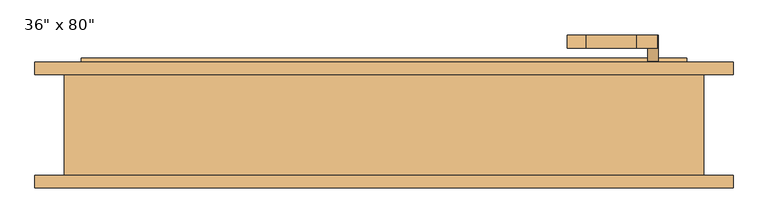
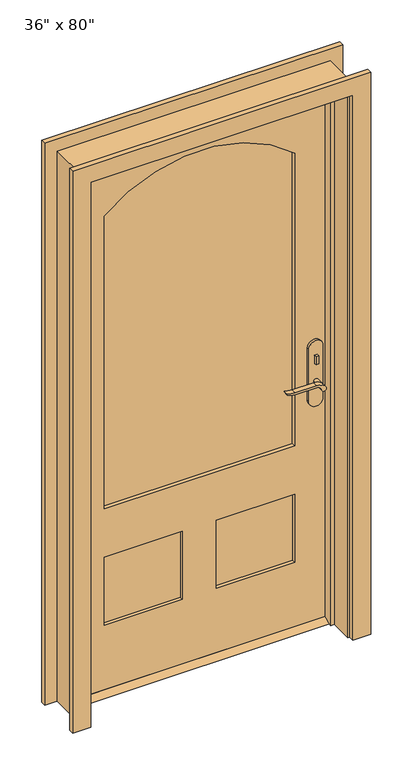
"""IFC4 building model written with IfcOpenShell, lengths in millimetres: door geometry."""

from ifc_helpers import new_model, si_unit, point, frame, frame_2d, origin, place, context, project, spatial, polyline, circle_curve, trimmed, segment, composite_curve, outline, extrude, faceted_brep, source, transform, mapped, element, save


def door_808aeb8e(model_context):
    return source(origin(), model_context, "Body", "SolidModel", [
        extrude(outline(polyline([(38.1, 12.7), (73.025, 12.7), (98.425, 0.0), (12.7, 0.0), (38.1, 12.7)])), frame((-457.2, 0.0, 0.0), z_axis=(1.0, 0.0, 0.0), x_axis=(0.0, 1.0, 0.0)), (0.0, 0.0, 1.0), 914.4),
        extrude(outline(polyline([(411.4, 18.1), (401.4, 18.1), (401.4, 28.1), (411.4, 28.1), (411.4, 18.1)])), frame((0.0, 0.0, 981.9), z_axis=(0.0, 0.0, 1.0), x_axis=(1.0, 0.0, 0.0)), (0.0, 0.0, 1.0), 30.0),
        extrude(outline(composite_curve([segment(trimmed(circle_curve(frame_2d((996.9, 406.4)), 8.0), [point((996.9, 398.4))], [point((996.9, 414.4))], False, "CARTESIAN"), True, "CONTINUOUS"), segment(trimmed(circle_curve(frame_2d((996.9, 406.4)), 8.0), [point((996.9, 414.4))], [point((996.9, 398.4))], False, "CARTESIAN"), True, "CONTINUOUS")], self_intersect=False)), frame((0.0, 83.025, 0.0), z_axis=(0.0, 1.0, 0.0), x_axis=(0.0, 0.0, 1.0)), (0.0, 0.0, 1.0), 10.0),
        extrude(outline(composite_curve([segment(trimmed(circle_curve(frame_2d((897.1555521, 382.7324871)), 37.2832219), [point((919.0523287, 412.9081363))], [point((934.4, 381.0325667))], False, "CARTESIAN"), True, "CONTINUOUS"), segment(polyline([(934.4, 381.0325667), (934.4, 304.7564091)]), True, "CONTINUOUS"), segment(trimmed(circle_curve(frame_2d((1017.6850638, 304.8227909)), 83.2850902), [point((934.4, 304.7564091))], [point((939.4, 276.4))], True, "CARTESIAN"), True, "CONTINUOUS"), segment(polyline([(939.4, 276.4), (936.6135558, 276.4)]), True, "CONTINUOUS"), segment(trimmed(circle_curve(frame_2d((986.6709207, 308.3396612)), 59.3791355), [point((936.6135558, 276.4))], [point((927.4, 304.7564091))], False, "CARTESIAN"), True, "CONTINUOUS"), segment(polyline([(927.4, 304.7564091), (927.4, 381.0138099)]), True, "CONTINUOUS"), segment(trimmed(circle_curve(frame_2d((909.2738613, 381.0138099)), 18.1261387), [point((927.4, 381.0138099))], [point((914.4, 398.4))], True, "CARTESIAN"), True, "CONTINUOUS"), segment(trimmed(circle_curve(frame_2d((914.4, 406.4)), 8.0), [point((914.4, 398.4))], [point((919.0523287, 412.9081363))], False, "CARTESIAN"), True, "CONTINUOUS")], self_intersect=False)), frame((0.0, -21.9, 0.0), z_axis=(0.0, 1.0, 0.0), x_axis=(0.0, 0.0, 1.0)), (0.0, 0.0, 1.0), 20.0),
        extrude(outline(composite_curve([segment(trimmed(circle_curve(frame_2d((914.4, 406.4)), 8.0), [point((914.3999903, 398.4))], [point((919.0523287, 412.9081363))], False, "CARTESIAN"), True, "CONTINUOUS"), segment(trimmed(circle_curve(frame_2d((897.1555521, 382.7324871)), 37.2832219), [point((919.0523287, 412.9081363))], [point((934.4, 381.0325667))], False, "CARTESIAN"), True, "CONTINUOUS"), segment(polyline([(934.4, 381.0325667), (934.4, 304.7564091)]), True, "CONTINUOUS"), segment(trimmed(circle_curve(frame_2d((1017.6850638, 304.8227909)), 83.2850902), [point((934.4, 304.7564091))], [point((939.4, 276.4))], True, "CARTESIAN"), True, "CONTINUOUS"), segment(polyline([(939.4, 276.4), (936.6135558, 276.4)]), True, "CONTINUOUS"), segment(trimmed(circle_curve(frame_2d((986.6709207, 308.3396612)), 59.3791355), [point((936.6135558, 276.4))], [point((927.4, 304.7564091))], False, "CARTESIAN"), True, "CONTINUOUS"), segment(polyline([(927.4, 304.7564091), (927.4, 381.0138122)]), True, "CONTINUOUS"), segment(trimmed(circle_curve(frame_2d((909.2738682, 381.0138122)), 18.1261318), [point((927.4, 381.0138122))], [point((914.3999903, 398.4))], True, "CARTESIAN"), True, "CONTINUOUS")], self_intersect=False)), frame((0.0, 113.025, 0.0), z_axis=(0.0, 1.0, 0.0), x_axis=(0.0, 0.0, 1.0)), (0.0, 0.0, 1.0), 20.0),
        extrude(outline(composite_curve([segment(trimmed(circle_curve(frame_2d((914.4, 406.4)), 8.0), [point((914.4, 398.4))], [point((914.4, 414.4))], False, "CARTESIAN"), True, "CONTINUOUS"), segment(trimmed(circle_curve(frame_2d((914.4, 406.4)), 8.0), [point((914.4, 414.4))], [point((914.4, 398.4))], False, "CARTESIAN"), True, "CONTINUOUS")], self_intersect=False)), frame((0.0, -1.9, 0.0), z_axis=(0.0, 1.0, 0.0), x_axis=(0.0, 0.0, 1.0)), (0.0, 0.0, 1.0), 30.0),
        extrude(outline(composite_curve([segment(trimmed(circle_curve(frame_2d((914.4, 406.4)), 8.0), [point((914.4, 398.4))], [point((914.4, 414.4))], False, "CARTESIAN"), True, "CONTINUOUS"), segment(trimmed(circle_curve(frame_2d((914.4, 406.4)), 8.0), [point((914.4, 414.4))], [point((914.4, 398.4))], False, "CARTESIAN"), True, "CONTINUOUS")], self_intersect=False)), frame((0.0, 83.025, 0.0), z_axis=(0.0, 1.0, 0.0), x_axis=(0.0, 0.0, 1.0)), (0.0, 0.0, 1.0), 30.0),
        extrude(outline(composite_curve([segment(polyline([(844.4, 431.4), (1039.4, 431.4)]), True, "CONTINUOUS"), segment(trimmed(circle_curve(frame_2d((1039.4, 406.4)), 25.0), [point((1039.4, 431.4))], [point((1039.4, 381.4))], False, "CARTESIAN"), True, "CONTINUOUS"), segment(polyline([(1039.4, 381.4), (844.4, 381.4)]), True, "CONTINUOUS"), segment(trimmed(circle_curve(frame_2d((844.4, 406.4)), 25.0), [point((844.4, 381.4))], [point((844.4, 431.4))], False, "CARTESIAN"), True, "CONTINUOUS")], self_intersect=False)), frame((0.0, 28.1, 0.0), z_axis=(0.0, 1.0, 0.0), x_axis=(0.0, 0.0, 1.0)), (0.0, 0.0, 1.0), 10.0),
        extrude(outline(composite_curve([segment(polyline([(844.4, 431.4), (1039.4, 431.4)]), True, "CONTINUOUS"), segment(trimmed(circle_curve(frame_2d((1039.4, 406.4)), 25.0), [point((1039.4, 431.4))], [point((1039.4, 381.4))], False, "CARTESIAN"), True, "CONTINUOUS"), segment(polyline([(1039.4, 381.4), (844.4, 381.4)]), True, "CONTINUOUS"), segment(trimmed(circle_curve(frame_2d((844.4, 406.4)), 25.0), [point((844.4, 381.4))], [point((844.4, 431.4))], False, "CARTESIAN"), True, "CONTINUOUS")], self_intersect=False)), frame((0.0, 73.025, 0.0), z_axis=(0.0, 1.0, 0.0), x_axis=(0.0, 0.0, 1.0)), (0.0, 0.0, 1.0), 10.0),
        extrude(outline(polyline([(2032.0, -457.2), (12.7, -457.2), (12.7, 457.2), (2032.0, 457.2), (2032.0, -457.2)]), holes=[composite_curve([segment(polyline([(688.975, -336.55), (1784.35, -336.55)]), True, "CONTINUOUS"), segment(trimmed(circle_curve(frame_2d((1401.92125, 0.0)), 509.42875), [point((1784.35, -336.55))], [point((1784.35, 336.55))], True, "CARTESIAN"), True, "CONTINUOUS"), segment(polyline([(1784.35, 336.55), (688.975, 336.55), (688.975, -336.55)]), True, "CONTINUOUS")], self_intersect=False), polyline([(508.0, -60.325), (254.0, -60.325), (254.0, -336.55), (508.0, -336.55), (508.0, -60.325)]), polyline([(508.0, 336.55), (254.0, 336.55), (254.0, 60.325), (508.0, 60.325), (508.0, 336.55)])]), frame((0.0, 38.1, 0.0), z_axis=(0.0, 1.0, 0.0), x_axis=(0.0, 0.0, 1.0)), (0.0, 0.0, 1.0), 34.925),
        faceted_brep([(482.6, 73.025, 0.0), (482.6, -79.375, 0.0), (457.2, -79.375, 0.0), (457.2, 3.175, 0.0), (444.5, 3.175, 0.0), (444.5, 38.1, 0.0), (457.2, 38.1, 0.0), (457.2, 73.025, 0.0), (482.6, 73.025, 2057.4), (482.6, -79.375, 2057.4), (-482.6, -79.375, 2057.4), (-482.6, -79.375, 0.0), (-457.2, -79.375, 0.0), (-457.2, -79.375, 2032.0), (457.2, -79.375, 2032.0), (457.2, 3.175, 2032.0), (-457.2, 3.175, 2032.0), (-457.2, 3.175, 0.0), (-444.5, 3.175, 0.0), (-444.5, 3.175, 2019.3), (444.5, 3.175, 2019.3), (444.5, 38.1, 2019.3), (-444.5, 38.1, 2019.3), (-444.5, 38.1, 0.0), (-457.2, 38.1, 0.0), (-457.2, 38.1, 2032.0), (457.2, 38.1, 2032.0), (457.2, 73.025, 2032.0), (-457.2, 73.025, 2032.0), (-457.2, 73.025, 0.0), (-482.6, 73.025, 0.0), (-482.6, 73.025, 2057.4)], [[[0, 1, 2, 3, 4, 5, 6, 7]], [[1, 0, 8, 9]], [[2, 1, 9, 10, 11, 12, 13, 14]], [[3, 2, 14, 15]], [[4, 3, 15, 16, 17, 18, 19, 20]], [[5, 4, 20, 21]], [[6, 5, 21, 22, 23, 24, 25, 26]], [[7, 6, 26, 27]], [[0, 7, 27, 28, 29, 30, 31, 8]], [[9, 8, 31, 10]], [[15, 14, 13, 16]], [[21, 20, 19, 22]], [[27, 26, 25, 28]], [[30, 29, 24, 23, 18, 17, 12, 11]], [[10, 31, 30, 11]], [[16, 13, 12, 17]], [[22, 19, 18, 23]], [[28, 25, 24, 29]]]),
        extrude(outline(polyline([(-60.325, 49.7416667), (-336.55, 49.7416667), (-336.55, 61.3833333), (-60.325, 61.3833333), (-60.325, 49.7416667)])), frame((0.0, 0.0, 254.0), z_axis=(0.0, 0.0, 1.0), x_axis=(1.0, 0.0, 0.0)), (0.0, 0.0, 1.0), 254.0),
        extrude(outline(polyline([(336.55, 49.7416667), (60.325, 49.7416667), (60.325, 61.3833333), (336.55, 61.3833333), (336.55, 49.7416667)])), frame((0.0, 0.0, 254.0), z_axis=(0.0, 0.0, 1.0), x_axis=(1.0, 0.0, 0.0)), (0.0, 0.0, 1.0), 254.0),
        extrude(outline(composite_curve([segment(polyline([(688.975, -336.55), (688.975, 336.55), (1784.35, 336.55)]), True, "CONTINUOUS"), segment(trimmed(circle_curve(frame_2d((1401.92125, 0.0)), 509.42875), [point((1784.35, 336.55))], [point((1784.35, -336.55))], False, "CARTESIAN"), True, "CONTINUOUS"), segment(polyline([(1784.35, -336.55), (688.975, -336.55)]), True, "CONTINUOUS")], self_intersect=False)), frame((0.0, 52.07, 0.0), z_axis=(0.0, 1.0, 0.0), x_axis=(0.0, 0.0, 1.0)), (0.0, 0.0, 1.0), 6.985),
        extrude(outline(polyline([(0.0, -527.05), (0.0, -463.55), (2038.35, -463.55), (2038.35, 463.55), (0.0, 463.55), (0.0, 527.05), (2101.85, 527.05), (2101.85, -527.05), (0.0, -527.05)])), frame((0.0, -98.425, 0.0), z_axis=(0.0, 1.0, 0.0), x_axis=(0.0, 0.0, 1.0)), (0.0, 0.0, 1.0), 19.05),
        extrude(outline(polyline([(0.0, -527.05), (0.0, -463.55), (2038.35, -463.55), (2038.35, 463.55), (0.0, 463.55), (0.0, 527.05), (2101.85, 527.05), (2101.85, -527.05), (0.0, -527.05)])), frame((0.0, 73.025, 0.0), z_axis=(0.0, 1.0, 0.0), x_axis=(0.0, 0.0, 1.0)), (0.0, 0.0, 1.0), 19.05),
    ])


if __name__ == "__main__":
    model = new_model("IFC4")
    model_context = context("Model", 3, world=origin())
    ifc_project = project(units=[si_unit("LENGTHUNIT", "METRE", prefix="MILLI")], contexts=[model_context])
    site = spatial("IfcSite", under=ifc_project)
    building = spatial("IfcBuilding", under=site)
    placement = place(None, origin())
    door_shape = door_808aeb8e(model_context)
    element("IfcDoor", 1, ObjectType="36\" x 80\"", at=placement, inside=building, context=model_context, shape_type="MappedRepresentation", body=[
        mapped(door_shape, transform((0.0, 0.0, 0.0), x_axis=(1.0, 0.0, 0.0), y_axis=(0.0, 1.0, 0.0), z_axis=(0.0, 0.0, 1.0))),
    ])
    save(model, "model.ifc")

# Revit data of these elements
# Type "36\" x 80\""
#   Type Mark = "9"
#   Assembly Code = "B2030100"
#   Analytic Construction = "French door, wood frame with single glass"
#   Threshold Offset [instance default] = 0' - 0 1/2"
#   Thickness = 0' - 1 3/8"
#   Thermal Resistance (R) = 1.0696 (h·ft²·°F)/BTU
#   Swing Angle [instance default] = 90.00°
#   Stiles = 0' - 4 3/4"
#   Rough Width = 3' - 2"
#   Rough Height = 6' - 9"
#   Radius = 1' - 8.05625"
#   Lock Rail = 0' - 7 1/8"
#   Height = 6' - 8"
#   Width = 3' - 0"
#   Heat Transfer Coefficient (U) = 0.9350 BTU/(h·ft²·°F)
#   Door Offset [instance default] = 0' - 0"
#   Bottom Rail = 0' - 9 1/2"
#   Threshold [instance default] = yes
#   Function = 1
#   Exterior Trim [instance default] = yes
#   Trim Material = Cherry
#   Threshold Material = Cherry
#   Panel Material = Cherry
#   Glazing = Glass
#   Frame Material = Cherry
#   Door Handle Material = Aluminum
#   Visual Light Transmittance = 0
#   Solar Heat Gain Coefficient = 0
#   Wall Closure = (empty or 0)
#   Construction Type = (empty or 0)
# Element 1 (IfcDoor, "36\" x 80\"")
#   Materials on its faces: "Cherry", "Aluminum", "Glass"
# Materials
#   "Cherry": class "Wood", colour RGB 226 177 128, transparency 0, Description = "Prunus Serotina", Cost = 0
#   "Glass": class "Glass", colour RGB 0 128 192, transparency 0.75, Description = "Soda Lime Glass", Cost = 0
#   "Aluminum": class "Metal", colour RGB 247 247 247, transparency 0, Description = "Aluminum 6061", Cost = 0
